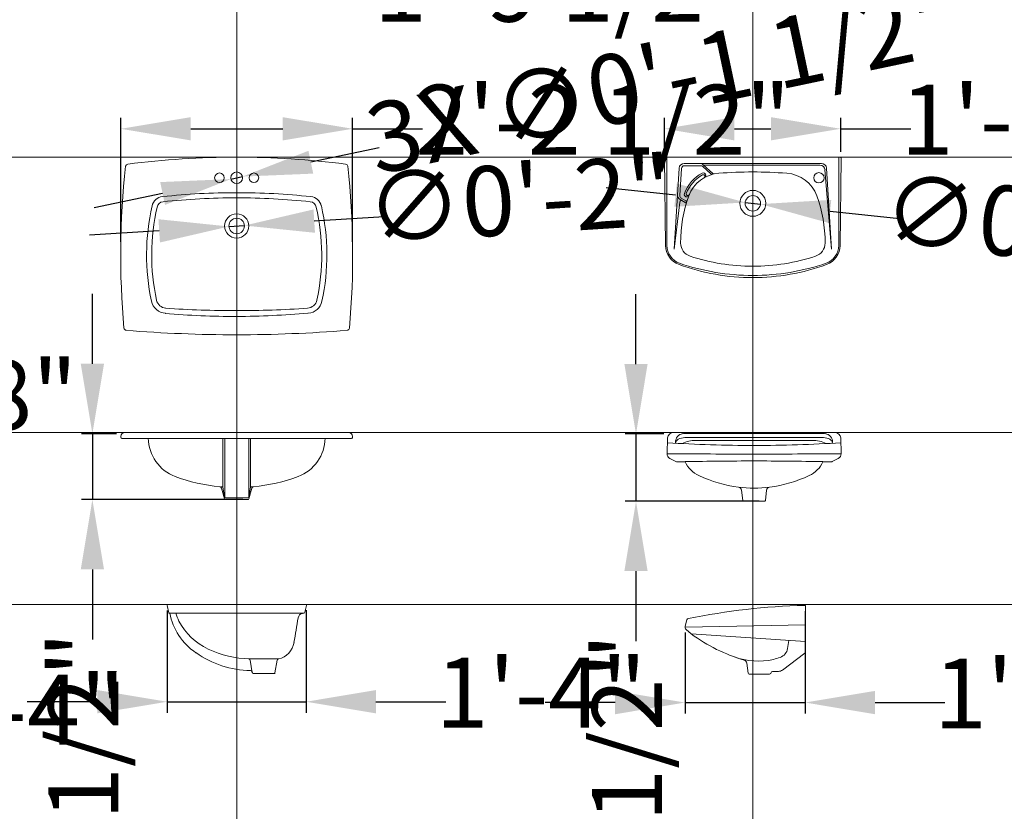
# Model space of a CAD drawing. Units: inches. Extents: x 2138 to 3265, y 2149 to 3392.
# Tile 11 of 13: x 3040 to 3153, y 3164 to 3255. Entities that reach past the tile are written whole.
import ezdxf

# ---------------------------------------------------------------- set-up
doc = ezdxf.new("R2010")
doc.units = ezdxf.units.IN
for name, color, linetype, lineweight in [('A-ANNO-DIMS', 2, 'Continuous', 18), ('A-DETL-GRID', 1, 'Continuous', 13), ('Washbasin-detail', 251, 'Continuous', 13), ('Washbasin-outline', 250, 'Continuous', 20)]:
    doc.layers.add(name, color=color, linetype=linetype, lineweight=lineweight)
doc.styles.get("Standard").update_dxf_attribs({"font": 'arial.ttf'})
doc.dimstyles.new('ISO-25', dxfattribs={"dimtxt": 8, "dimasz": 8, "dimexe": 1.25, "dimexo": 0.625, "dimtad": 0, "dimdec": 1, "dimlunit": 4, "dimtxsty": 'Standard', "dimcen": 2.5, "dimadec": 0, "dimazin": 0, "dimtfac": 1, "dimtdec": 1, "dimtmove": 0, "dimatfit": 3, "dimfxl": 1, "dimarcsym": 0})

# ---------------------------------------------------------------- blocks, each defined once
blk = doc.blocks.new('*D72')
at = {"layer": 'A-ANNO-DIMS', "color": 0, "lineweight": -2, "transparency": 16777216}
for p, q in [((3073.65, 3297.38), (3073.65, 3256.24)), ((3052.31, 3294.65), (3052.31, 3256.24)), ((3060.31, 3257.49), (3065.65, 3257.49)), ((3073.65, 3257.49), (3081.65, 3257.49))]:
    blk.add_line(p, q, dxfattribs=at)
at = {"layer": 'A-ANNO-DIMS', "color": 0, "transparency": 16777216}
for points in [[(3060.31, 3258.82), (3060.31, 3256.15), (3052.31, 3257.49)], [(3065.65, 3258.82), (3065.65, 3256.15), (3073.65, 3257.49)]]:
    blk.add_solid(points, dxfattribs=at)
at = {"layer": 'Defpoints', "color": 0, "transparency": 16777216}
for p in [(3073.65, 3298.01), (3052.31, 3295.28), (3073.65, 3257.49)]:
    blk.add_point(p, dxfattribs=at)
at = {"layer": 'A-ANNO-DIMS', "color": 0, "transparency": 16777216, "insert": (3101.86, 3257.49), "char_height": 8, "attachment_point": 5}
blk.add_mtext('1\'-9 1/2"', dxfattribs=at)
blk = doc.blocks.new('*D85')
at = {"layer": 'A-ANNO-DIMS', "color": 0, "lineweight": -2, "transparency": 16777216}
for p, q in [((2995.75, 3208.1), (2995.75, 3212.02)), ((3015.52, 3208.08), (3015.52, 3212.02)), ((3003.75, 3210.77), (3007.52, 3210.77)), ((3015.52, 3210.77), (3023.52, 3210.77))]:
    blk.add_line(p, q, dxfattribs=at)
at = {"layer": 'A-ANNO-DIMS', "color": 0, "transparency": 16777216}
for points in [[(3003.75, 3212.11), (3003.75, 3209.44), (2995.75, 3210.77)], [(3007.52, 3212.11), (3007.52, 3209.44), (3015.52, 3210.77)]]:
    blk.add_solid(points, dxfattribs=at)
at = {"layer": 'Defpoints', "color": 0, "transparency": 16777216}
for p in [(3015.52, 3210.77), (2995.75, 3207.48), (3015.52, 3207.45)]:
    blk.add_point(p, dxfattribs=at)
at = {"layer": 'A-ANNO-DIMS', "color": 0, "transparency": 16777216, "insert": (3034.4, 3210.77), "char_height": 8, "attachment_point": 5}
blk.add_mtext('1\'-8"', dxfattribs=at)
blk = doc.blocks.new('*D87')
at = {"layer": 'A-ANNO-DIMS', "color": 0, "lineweight": -2, "transparency": 16777216}
for p, q in [((3012.99, 3186.82), (3012.99, 3173.53)), ((2997.1, 3184.61), (2997.1, 3173.53)), ((2989.1, 3174.78), (2981.1, 3174.78)), ((2997.1, 3174.78), (3012.99, 3174.78)), ((3020.99, 3174.78), (3028.99, 3174.78))]:
    blk.add_line(p, q, dxfattribs=at)
at = {"layer": 'A-ANNO-DIMS', "color": 0, "transparency": 16777216}
for points in [[(2989.1, 3176.11), (2989.1, 3173.44), (2997.1, 3174.78)], [(3020.99, 3176.11), (3020.99, 3173.44), (3012.99, 3174.78)]]:
    blk.add_solid(points, dxfattribs=at)
at = {"layer": 'Defpoints', "color": 0, "transparency": 16777216}
for p in [(3012.99, 3187.44), (2997.1, 3185.23), (3012.99, 3174.78)]:
    blk.add_point(p, dxfattribs=at)
at = {"layer": 'A-ANNO-DIMS', "color": 0, "transparency": 16777216, "insert": (3039.87, 3174.78), "char_height": 8, "attachment_point": 5}
blk.add_mtext('1\'-4"', dxfattribs=at)
blk = doc.blocks.new('*D88')
at = {"layer": 'A-ANNO-DIMS', "color": 0, "lineweight": -2, "transparency": 16777216}
for p, q in [((3051.42, 3229.35), (3051.42, 3243.52)), ((3077.95, 3229.35), (3077.95, 3243.52)), ((3059.42, 3242.27), (3069.95, 3242.27)), ((3077.95, 3242.27), (3085.95, 3242.27))]:
    blk.add_line(p, q, dxfattribs=at)
at = {"layer": 'A-ANNO-DIMS', "color": 0, "transparency": 16777216}
for points in [[(3059.42, 3243.6), (3059.42, 3240.94), (3051.42, 3242.27)], [(3069.95, 3243.6), (3069.95, 3240.94), (3077.95, 3242.27)]]:
    blk.add_solid(points, dxfattribs=at)
at = {"layer": 'Defpoints', "color": 0, "transparency": 16777216}
for p in [(3077.95, 3242.27), (3051.42, 3228.73), (3077.95, 3228.73)]:
    blk.add_point(p, dxfattribs=at)
at = {"layer": 'A-ANNO-DIMS', "color": 0, "transparency": 16777216, "insert": (3106.59, 3242.27), "char_height": 8, "attachment_point": 5}
blk.add_mtext('2\'-2 1/2"', dxfattribs=at)
blk = doc.blocks.new('*D89')
at = {"layer": 'A-ANNO-DIMS', "color": 0, "lineweight": -2, "transparency": 16777216}
for p, q in [((3048.17, 3215.38), (3048.17, 3223.38)), ((3050.93, 3207.38), (3046.92, 3207.38)), ((3048.17, 3207.38), (3048.17, 3199.85)), ((3065.38, 3199.85), (3046.92, 3199.85)), ((3048.17, 3191.85), (3048.17, 3183.85))]:
    blk.add_line(p, q, dxfattribs=at)
at = {"layer": 'A-ANNO-DIMS', "color": 0, "transparency": 16777216}
for points in [[(3046.84, 3215.38), (3049.5, 3215.38), (3048.17, 3207.38)], [(3046.84, 3191.85), (3049.5, 3191.85), (3048.17, 3199.85)]]:
    blk.add_solid(points, dxfattribs=at)
at = {"layer": 'Defpoints', "color": 0, "transparency": 16777216}
for p in [(3051.56, 3207.38), (3048.17, 3199.85), (3066, 3199.85)]:
    blk.add_point(p, dxfattribs=at)
at = {"layer": 'A-ANNO-DIMS', "color": 0, "transparency": 16777216, "insert": (3048.17, 3163.27), "char_height": 8, "attachment_point": 5, "rotation": 90}
blk.add_mtext('0\'-7 1/2"', dxfattribs=at)
blk = doc.blocks.new('*D90')
at = {"layer": 'A-ANNO-DIMS', "color": 0, "lineweight": -2, "transparency": 16777216}
for p, q in [((3056.72, 3187.14), (3056.72, 3175.46)), ((3072.62, 3187.18), (3072.62, 3175.46)), ((3048.72, 3176.71), (3040.72, 3176.71)), ((3056.72, 3176.71), (3072.62, 3176.71)), ((3080.62, 3176.71), (3088.62, 3176.71))]:
    blk.add_line(p, q, dxfattribs=at)
at = {"layer": 'A-ANNO-DIMS', "color": 0, "transparency": 16777216}
for points in [[(3048.72, 3178.05), (3048.72, 3175.38), (3056.72, 3176.71)], [(3080.62, 3178.05), (3080.62, 3175.38), (3072.62, 3176.71)]]:
    blk.add_solid(points, dxfattribs=at)
at = {"layer": 'Defpoints', "color": 0, "transparency": 16777216}
for p in [(3056.72, 3187.77), (3072.62, 3187.8), (3072.62, 3176.71)]:
    blk.add_point(p, dxfattribs=at)
at = {"layer": 'A-ANNO-DIMS', "color": 0, "transparency": 16777216, "insert": (3099.5, 3176.71), "char_height": 8, "attachment_point": 5}
blk.add_mtext('1\'-4"', dxfattribs=at)
blk = doc.blocks.new('*D91')
at = {"layer": 'A-ANNO-DIMS', "color": 0, "lineweight": -2, "transparency": 16777216}
for p, q in [((3113.64, 3239.59), (3113.64, 3243.52)), ((3133.8, 3239.62), (3133.8, 3243.52)), ((3121.64, 3242.27), (3125.8, 3242.27)), ((3133.8, 3242.27), (3141.8, 3242.27))]:
    blk.add_line(p, q, dxfattribs=at)
at = {"layer": 'A-ANNO-DIMS', "color": 0, "transparency": 16777216}
for points in [[(3121.64, 3243.6), (3121.64, 3240.94), (3113.64, 3242.27)], [(3125.8, 3243.6), (3125.8, 3240.94), (3133.8, 3242.27)]]:
    blk.add_solid(points, dxfattribs=at)
at = {"layer": 'Defpoints', "color": 0, "transparency": 16777216}
for p in [(3133.8, 3242.27), (3113.64, 3238.97), (3133.8, 3239)]:
    blk.add_point(p, dxfattribs=at)
at = {"layer": 'A-ANNO-DIMS', "color": 0, "transparency": 16777216, "insert": (3152.69, 3242.27), "char_height": 8, "attachment_point": 5}
blk.add_mtext('1\'-8"', dxfattribs=at)
blk = doc.blocks.new('*D92')
at = {"layer": 'A-ANNO-DIMS', "color": 0, "lineweight": -2, "transparency": 16777216}
for p, q in [((3110.37, 3215.35), (3110.37, 3223.35)), ((3113.57, 3207.35), (3109.12, 3207.35)), ((3110.37, 3207.35), (3110.37, 3199.66)), ((3124.47, 3199.66), (3109.12, 3199.66)), ((3110.37, 3191.66), (3110.37, 3183.66))]:
    blk.add_line(p, q, dxfattribs=at)
at = {"layer": 'A-ANNO-DIMS', "color": 0, "transparency": 16777216}
for points in [[(3109.04, 3215.35), (3111.7, 3215.35), (3110.37, 3207.35)], [(3109.04, 3191.66), (3111.7, 3191.66), (3110.37, 3199.66)]]:
    blk.add_solid(points, dxfattribs=at)
at = {"layer": 'Defpoints', "color": 0, "transparency": 16777216}
for p in [(3114.19, 3207.35), (3110.37, 3199.66), (3125.1, 3199.66)]:
    blk.add_point(p, dxfattribs=at)
at = {"layer": 'A-ANNO-DIMS', "color": 0, "transparency": 16777216, "insert": (3110.37, 3163.08), "char_height": 8, "attachment_point": 5, "rotation": 90}
blk.add_mtext('0\'-7 1/2"', dxfattribs=at)
blk = doc.blocks.new('*D93')
at = {"layer": 'A-ANNO-DIMS', "color": 0, "lineweight": -2, "transparency": 16777216}
for p, q in [((3129.72, 3187.08), (3129.72, 3175.37)), ((3115.98, 3184.63), (3115.98, 3175.37)), ((3107.98, 3176.62), (3099.98, 3176.62)), ((3115.98, 3176.62), (3129.72, 3176.62)), ((3137.72, 3176.62), (3145.72, 3176.62))]:
    blk.add_line(p, q, dxfattribs=at)
at = {"layer": 'A-ANNO-DIMS', "color": 0, "transparency": 16777216}
for points in [[(3107.98, 3177.95), (3107.98, 3175.28), (3115.98, 3176.62)], [(3137.72, 3177.95), (3137.72, 3175.28), (3129.72, 3176.62)]]:
    blk.add_solid(points, dxfattribs=at)
at = {"layer": 'Defpoints', "color": 0, "transparency": 16777216}
for p in [(3129.72, 3187.71), (3115.98, 3185.26), (3129.72, 3176.62)]:
    blk.add_point(p, dxfattribs=at)
at = {"layer": 'A-ANNO-DIMS', "color": 0, "transparency": 16777216, "insert": (3165.92, 3176.62), "char_height": 8, "attachment_point": 5}
blk.add_mtext('1\'-1 1/2"', dxfattribs=at)
blk = doc.blocks.new('*D125')
at = {"layer": 'A-ANNO-DIMS', "color": 0, "lineweight": -2, "transparency": 16777216}
for p, q in [((3080.99, 3240.1), (3073.17, 3238.45)), ((3064.03, 3236.52), (3065.34, 3236.8)), ((3056.2, 3234.87), (3048.37, 3233.21))]:
    blk.add_line(p, q, dxfattribs=at)
at = {"layer": 'A-ANNO-DIMS', "color": 0, "transparency": 16777216}
for points in [[(3072.89, 3239.75), (3073.44, 3237.14), (3065.34, 3236.8)], [(3055.93, 3236.17), (3056.48, 3233.56), (3064.03, 3236.52)]]:
    blk.add_solid(points, dxfattribs=at)
at = {"layer": 'Defpoints', "color": 0, "transparency": 16777216}
for p in [(3065.34, 3236.8), (3064.03, 3236.52)]:
    blk.add_point(p, dxfattribs=at)
at = {"layer": 'A-ANNO-DIMS', "color": 0, "transparency": 16777216, "insert": (3113.58, 3246.98), "char_height": 8, "attachment_point": 5, "rotation": 11.9181}
blk.add_mtext('3X ∅0\'-1 1/2"', dxfattribs=at)
blk = doc.blocks.new('*D126')
at = {"layer": 'A-ANNO-DIMS', "color": 0, "lineweight": -2, "transparency": 16777216}
for p, q in [((3081.54, 3232.21), (3073.55, 3231.7)), ((3063.8, 3231.09), (3065.57, 3231.2)), ((3055.81, 3230.59), (3047.83, 3230.08))]:
    blk.add_line(p, q, dxfattribs=at)
at = {"layer": 'A-ANNO-DIMS', "color": 0, "transparency": 16777216}
for points in [[(3073.47, 3233.04), (3073.64, 3230.37), (3065.57, 3231.2)], [(3055.73, 3231.92), (3055.9, 3229.26), (3063.8, 3231.09)]]:
    blk.add_solid(points, dxfattribs=at)
at = {"layer": 'Defpoints', "color": 0, "transparency": 16777216}
for p in [(3063.8, 3231.09), (3065.57, 3231.2)]:
    blk.add_point(p, dxfattribs=at)
at = {"layer": 'A-ANNO-DIMS', "color": 0, "transparency": 16777216, "insert": (3097.11, 3233.19), "char_height": 8, "attachment_point": 5, "rotation": 3.6089}
blk.add_mtext('∅0\'-2"', dxfattribs=at)
blk = doc.blocks.new('*D127')
at = {"layer": 'A-ANNO-DIMS', "color": 0, "lineweight": -2, "transparency": 16777216}
for p, q in [((3114.9, 3234.67), (3106.94, 3235.51)), ((3122.86, 3233.84), (3124.62, 3233.65)), ((3140.53, 3231.98), (3132.58, 3232.81))]:
    blk.add_line(p, q, dxfattribs=at)
at = {"layer": 'A-ANNO-DIMS', "color": 0, "transparency": 16777216}
for points in [[(3115.04, 3236), (3114.76, 3233.35), (3122.86, 3233.84)], [(3132.71, 3234.14), (3132.44, 3231.49), (3124.62, 3233.65)]]:
    blk.add_solid(points, dxfattribs=at)
at = {"layer": 'Defpoints', "color": 0, "transparency": 16777216}
for p in [(3122.86, 3233.84), (3124.62, 3233.65)]:
    blk.add_point(p, dxfattribs=at)
at = {"layer": 'A-ANNO-DIMS', "color": 0, "transparency": 16777216, "insert": (3156.06, 3230.35), "char_height": 8, "attachment_point": 5, "rotation": 353.9986}
blk.add_mtext('∅0\'-2"', dxfattribs=at)

msp = doc.modelspace()

# ---------------------------------------------------------------- linework, layer by layer
at = {"layer": 'A-DETL-GRID'}
for p, q in [((3064.68, 3239.02), (3064.68, 3370.91)), ((3123.74, 3239.02), (3123.74, 3370.91)), ((2828.46, 3239.02), (3241.85, 3239.02)), ((2828.46, 3239.02), (3241.85, 3239.02)), ((3064.68, 3148.47), (3064.68, 3239.02)), ((3123.74, 3148.47), (3123.74, 3239.02)), ((2828.46, 3207.52), (3241.85, 3207.52)), ((2828.46, 3187.84), (3241.85, 3187.84))]:
    msp.add_line(p, q, dxfattribs=at)
at = {"layer": 'Washbasin-detail'}
for p, q in [((3113.9, 3239.02), (3113.9, 3228.9)), ((3133.58, 3239.02), (3133.58, 3228.9)), ((3123.74, 3238.31), (3115.9, 3238.31)), ((3117.79, 3238.04), (3115.9, 3238.04)), ((3118, 3237.95), (3118.93, 3237.1)), ((3118.07, 3238.16), (3119.16, 3237.16)), ((3131.41, 3238.11), (3118.11, 3238.11)), ((3123.74, 3238.31), (3131.58, 3238.31)), ((3114.75, 3228.51), (3115.31, 3237.76)), ((3115.39, 3234.63), (3115.58, 3237.74)), ((3132.73, 3228.51), (3131.99, 3237.57)), ((3132.73, 3228.51), (3132.17, 3237.76)), ((3115.38, 3233.89), (3114.75, 3228.51)), ((3115.42, 3234.19), (3116.01, 3233.85)), ((3115.55, 3234.34), (3116.07, 3234.04)), ((3123.88, 3207.41), (3115.91, 3207.41)), ((3123.88, 3207.41), (3131.85, 3207.41)), ((3063.11, 3206.85), (3063.11, 3201.3)), ((3063.31, 3206.85), (3063.31, 3200.1)), ((3066.06, 3206.85), (3066.06, 3200.1)), ((3066.25, 3206.85), (3066.25, 3201.3)), ((3114.89, 3206.42), (3114.89, 3206.29)), ((3123.88, 3206.93), (3115.95, 3206.93)), ((3117.21, 3206.62), (3130.55, 3206.62)), ((3123.88, 3206.93), (3131.81, 3206.93)), ((3062.82, 3201.29), (3063.11, 3201.29)), ((3063.29, 3199.93), (3062.96, 3201.13)), ((3063.11, 3201.28), (3063.29, 3200.14)), ((3066.25, 3201.28), (3066.07, 3200.14)), ((3066.08, 3199.93), (3066.41, 3201.13)), ((3066.55, 3201.29), (3066.25, 3201.29)), ((3063.4, 3199.85), (3064.68, 3199.85)), ((3063.41, 3200.04), (3064.69, 3200.04)), ((3063.41, 3200.04), (3064.69, 3200.04)), ((3065.95, 3200.04), (3064.68, 3200.04)), ((3065.95, 3200.04), (3064.68, 3200.04)), ((3065.97, 3199.85), (3064.68, 3199.85)), ((3129.76, 3185.5), (3115.98, 3185.26)), ((3116.69, 3184.47), (3129.76, 3183.61)), ((3127.87, 3183.73), (3127.72, 3182.8))]:
    msp.add_line(p, q, dxfattribs=at)
for centre, radius in [((3062.71, 3236.66), 0.551), ((3064.68, 3236.66), 0.669), ((3066.65, 3236.66), 0.551), ((3131.3, 3236.66), 0.591)]:
    msp.add_circle(centre, radius, dxfattribs=at)
for centre, radius, start, end in [((3115.9, 3237.72), 0.591, 90, 176.5501), ((3115.9, 3237.72), 0.315, 90, 176.5501), ((3117.67, 3237.72), 0.591, 47.5081, 90), ((3117.79, 3237.72), 0.315, 47.5081, 90), ((3131.41, 3237.52), 0.591, 4.6212, 90), ((3131.58, 3237.72), 0.591, 3.4499, 90), ((3120.14, 3233.25), 4.53, 119.1249, 158.9278), ((3120.14, 3233.25), 4.33, 119.974, 157.8804), ((3118.08, 3236.95), 0.289, 298.884, 120.9504), ((3118.07, 3236.83), 0.19, 299.8578, 119.974), ((3119.06, 3237.25), 0.197, 227.5081, 284.9221), ((3119.29, 3237.3), 0.197, 227.5081, 281.6214), ((3115.71, 3234.7), 0.591, 176.5501, 239.9947), ((3115.71, 3234.61), 0.315, 176.5501, 239.9947), ((3116.18, 3234.76), 0.287, 157.239, 339.7253), ((3116.3, 3234.81), 0.189, 157.8804, 337.9006), ((3123.74, 3233.74), 1.48, 90, 270), ((3123.74, 3233.74), 0.886, 90, 270), ((3123.74, 3233.74), 1.48, 270, 90), ((3123.74, 3233.74), 0.886, 270, 90), ((3079.63, 3227.83), 24.67, 167.1604, 192.0964), ((3056.34, 3233.14), 0.787, 96.1416, 167.1604), ((3064.68, 3155.63), 78.74, 90, 96.1416), ((3064.68, 3155.63), 78.74, 83.8584, 90), ((3073.02, 3233.14), 0.787, 12.8396, 83.8584), ((3049.74, 3227.83), 24.67, 347.9251, 12.8396), ((3115.58, 3233.87), 0.197, 59.9947, 173.2749), ((3115.91, 3233.68), 0.197, 343.7163, 59.9947), ((3115.97, 3233.87), 0.197, 342.9893, 59.9947), ((3064.68, 3231.15), 1.38, 90, 270), ((3064.68, 3231.15), 1.38, 270, 90), ((3064.68, 3231.15), 0.886, 90, 270), ((3064.68, 3231.15), 0.886, 270, 90), ((3116.12, 3228.96), 2.22, 180.7821, 249.7803), ((3131.36, 3228.96), 2.22, 290.2197, 359.2179), ((3123.74, 3251.47), 25.98, 251.1623, 270), ((3123.74, 3251.47), 25.98, 270, 288.8377), ((3056.66, 3222.92), 1.18, 192.0749, 266.0653), ((3072.71, 3222.92), 1.18, 273.9347, 347.9251), ((3064.68, 3339.57), 118.11, 266.049, 270), ((3064.68, 3339.57), 118.11, 270, 273.9347), ((3115.91, 3206.22), 1.18, 90, 99.548), ((3131.85, 3206.22), 1.18, 80.452, 90), ((3059.29, 3206.91), 4.72, 180.6352, 249.5876), ((3070.07, 3206.91), 4.72, 290.4124, 359.3648), ((3115.87, 3206.42), 0.984, 99.548, 180), ((3115.48, 3206.22), 0.591, 118.4442, 173.4004), ((3115.95, 3205.36), 1.57, 90, 118.4442), ((3117.21, 3203.16), 3.46, 90, 116.7072), ((3130.55, 3203.16), 3.46, 63.2928, 90), ((3131.81, 3205.36), 1.57, 61.5558, 90), ((3131.88, 3206.42), 0.984, 0, 80.452), ((3132.28, 3206.22), 0.591, 6.5996, 61.5558), ((3123.88, 4523.81), 1318.76, 269.56724, 270), ((3123.88, 4523.81), 1318.76, 270, 270.43276), ((3064.65, 3221.3), 20.08, 249.5876, 264.5822), ((3064.72, 3221.3), 20.08, 275.4178, 290.4124), ((3062.73, 3201.07), 0.236, 15.2242, 84.5822), ((3063.23, 3201.3), 0.118, 180, 188.9509), ((3066.13, 3201.3), 0.118, 351.0491, 0), ((3066.63, 3201.07), 0.236, 95.4178, 164.7758), ((3063.41, 3200.16), 0.118, 188.9509, 270), ((3063.4, 3199.96), 0.118, 195.2242, 270), ((3065.95, 3200.16), 0.118, 270, 351.0491), ((3065.97, 3199.96), 0.118, 270, 344.7758), ((3063.98, 3188.2), 7.09, 190.9924, 235.973), ((3126.43, 3183.01), 1.3, 290.1504, 350.6185), ((3066.42, 3191.3), 11.02, 234.5166, 269.1523), ((3124.38, 3189.5), 8.14, 250.1072, 282.2031), ((3124.06, 3189.48), 8.19, 284.427, 290.1504)]:
    msp.add_arc(centre, radius, start, end, dxfattribs=at)
at = {"layer": 'Washbasin-outline'}
for p, q in [((3051.89, 3207.52), (3064.68, 3207.52)), ((3077.47, 3207.52), (3064.68, 3207.52)), ((3051.42, 3207.05), (3051.42, 3206.97)), ((3051.54, 3206.85), (3064.69, 3206.85)), ((3077.83, 3206.85), (3064.68, 3206.85)), ((3077.95, 3207.05), (3077.95, 3206.97)), ((3056.9, 3186.88), (3056.71, 3187.72)), ((3056.83, 3187.84), (3072.54, 3187.84)), ((3072.66, 3187.72), (3072.48, 3186.96)), ((3056.93, 3186.85), (3057.03, 3186.85)), ((3057.03, 3186.85), (3072.4, 3186.85)), ((3072.2, 3186.81), (3072.36, 3186.84)), ((3066.17, 3181.62), (3069.52, 3181.62)), ((3066.22, 3181.45), (3066.47, 3180.03)), ((3069.32, 3181.45), (3069.06, 3180.03)), ((3066.48, 3180.02), (3066.44, 3180.14)), ((3066.55, 3179.96), (3068.99, 3179.96))]:
    msp.add_line(p, q, dxfattribs=at)
for points in [[(3115.3, 3226.74, -0.310499), (3113.76, 3228.93), (3113.62, 3238.9, -0.418217), (3113.74, 3239.02), (3123.74, 3239.02), (3133.74, 3239.02, -0.418217), (3133.86, 3238.9), (3133.72, 3228.93, -0.310499), (3132.17, 3226.74, -0.088455), (3123.74, 3225.24, -0.088455)], [(3123.88, 3207.52), (3114.66, 3207.52, 0.377881), (3113.96, 3206.9), (3113.92, 3205.09, 0.28521), (3114.23, 3204.56), (3114.93, 3204.19, 0.126322), (3115.06, 3204.16, -0.000566), (3116, 3204.18, 0.184451), (3117.57, 3202.58, 0.073376), (3122.1, 3201.26, -0.338761), (3122.44, 3200.92), (3122.59, 3199.75, 0.377345), (3122.7, 3199.65), (3123.88, 3199.65), (3125.05, 3199.65, 0.377345), (3125.17, 3199.75), (3125.32, 3200.92, -0.338761), (3125.66, 3201.26, 0.073376), (3130.18, 3202.58, 0.184451), (3131.76, 3204.18, -0.000566), (3132.7, 3204.16, 0.126322), (3132.82, 3204.19), (3133.52, 3204.56, 0.28521), (3133.84, 3205.09), (3133.8, 3206.9, 0.377881), (3133.1, 3207.52)]]:
    msp.add_lwpolyline(points, format="xyb", close=True, dxfattribs=at)
msp.add_lwpolyline([(3126.08, 3180.18), (3126.66, 3180.18), (3126.08, 3180.18, 0.335437), (3125.78, 3179.95, -0.335437), (3125.66, 3179.87), (3123.31, 3179.87, -0.377345), (3123.19, 3179.97), (3123.04, 3181.14, 0.297687), (3122.76, 3181.47, -0.086663), (3116.69, 3184.47), (3116.12, 3184.96, -0.289634), (3115.99, 3185.36), (3116.18, 3186.07, -0.28455), (3116.36, 3186.24, -0.042482), (3129.64, 3187.74, -0.422344), (3129.76, 3187.62), (3129.76, 3182.41, -0.236068), (3129.68, 3182.25), (3127.13, 3180.34, -0.162278), (3126.66, 3180.18)], format="xyb", dxfattribs=at)
for centre, radius, start, end in [((3064.68, 3140.59), 98.43, 90, 97.2742), ((3064.68, 3140.59), 98.43, 82.7258, 90), ((3143.98, 3227.76), 92.57, 173.6587, 185.1425), ((3052.26, 3237.95), 0.276, 97.2742, 173.6587), ((3077.11, 3237.95), 0.276, 6.3413, 82.7258), ((2985.38, 3227.76), 92.57, 354.8575, 6.3413), ((3120.12, 3233.25), 3.94, 94.015, 159.961), ((3123.98, 3178.27), 59.06, 90.2363, 94.015), ((3123.49, 3178.27), 59.06, 85.985, 89.7637), ((3127.35, 3233.25), 3.94, 20.039, 85.985), ((3056.34, 3233.14), 1.38, 96.1416, 167.1604), ((3064.68, 3155.63), 79.33, 90, 96.1416), ((3064.68, 3155.63), 79.33, 83.8584, 90), ((3073.02, 3233.14), 1.38, 12.8396, 83.8584), ((3131.22, 3229.21), 15.75, 159.961, 180.0563), ((3116.26, 3229.21), 15.75, 359.9437, 20.039), ((3079.63, 3227.83), 25.26, 167.1604, 192.0749), ((3049.74, 3227.83), 25.26, 347.9251, 12.8396), ((3117.05, 3229.19), 1.57, 180, 251.6504), ((3130.43, 3229.19), 1.57, 288.3496, 0), ((3123.74, 3249.37), 22.83, 251.6504, 270), ((3123.74, 3249.37), 22.83, 270, 288.3496), ((3056.66, 3222.92), 1.77, 192.0749, 266.0653), ((3072.71, 3222.92), 1.77, 275.0575, 347.9251), ((3064.68, 3313.58), 92.79, 264.9425, 270), ((3063.54, 3339.49), 118.7, 270.5523, 274.5052), ((3072.71, 3222.92), 1.77, 273.9347, 275.0575), ((3052.06, 3219.49), 0.276, 185.1425, 265.3953), ((3064.68, 3376.18), 157.48, 265.3953, 270), ((3064.68, 3376.18), 157.48, 270, 274.6047), ((3077.3, 3219.49), 0.276, 274.6047, 354.8575), ((3051.89, 3207.05), 0.472, 90, 180), ((3077.47, 3207.05), 0.472, 0, 90), ((3051.54, 3206.97), 0.118, 180, 270), ((3077.83, 3206.97), 0.118, 270, 0), ((3123.88, 3358.99), 152.96, 266.2773, 270.0006), ((3123.88, 3358.99), 152.96, 269.9994, 273.7227), ((3123.88, 2789.3), 414.96, 90, 91.0879), ((3123.88, 2789.3), 414.96, 88.9121, 90), ((3123.88, 3215.22), 14.07, 262.7274, 277.2726), ((3056.83, 3187.72), 0.118, 90, 180), ((3072.54, 3187.72), 0.118, 0, 90), ((3056.94, 3186.89), 0.0394, 192.8043, 256.7595), ((3062.53, 3188.3), 5.04, 196.7804, 207.8951), ((2876.94, 3217.46), 197.24, 350.0842, 350.9161), ((3072.3, 3186.23), 0.591, 100.008, 170.9161), ((3072.33, 3186.99), 0.157, 280.008, 347.1957), ((3064.62, 3189.41), 7.4, 207.8951, 244.3062), ((3066.33, 3192.96), 11.34, 244.3062, 269.213), ((3068.92, 3183.9), 2.36, 283.4865, 350.0842), ((3066.03, 3181.41), 0.197, 10.1247, 76.5135), ((3069.51, 3181.41), 0.197, 103.4865, 169.8753), ((3066.25, 3180.08), 0.197, 17.354, 89.1523), ((3066.55, 3180.04), 0.0787, 197.354, 270), ((3068.99, 3180.04), 0.0787, 270, 349.8753)]:
    msp.add_arc(centre, radius, start, end, dxfattribs=at)

# ---------------------------------------------------------------- dimensions: what is measured, and where the dimension line sits
at = {"layer": 'A-ANNO-DIMS'}
for base, p1, p2, picture, middle in [((3073.65, 3257.49), (3052.31, 3295.28), (3073.65, 3298.01), '*D72', (3101.86, 3257.49)), ((3077.95, 3242.27), (3051.42, 3228.73), (3077.95, 3228.73), '*D88', (3106.59, 3242.27)), ((3133.8, 3242.27), (3113.64, 3238.97), (3133.8, 3239), '*D91', (3152.69, 3242.27)), ((3015.52, 3210.77), (2995.75, 3207.48), (3015.52, 3207.45), '*D85', (3034.4, 3210.77)), ((3129.72, 3176.62), (3115.98, 3185.26), (3129.72, 3187.71), '*D93', (3165.92, 3176.62)), ((3012.99, 3174.78), (2997.1, 3185.23), (3012.99, 3187.44), '*D87', (3039.87, 3174.78)), ((3072.62, 3176.71), (3056.72, 3187.77), (3072.62, 3187.8), '*D90', (3099.5, 3176.71))]:
    dim = msp.add_linear_dim(base=base, p1=p1, p2=p2, dimstyle='ISO-25', override={"dimdec": 1, "dimlfac": 1, "dimrnd": 0, "dimzin": 1, "dimdsep": 46, "dimlunit": 4, "dimfrac": 2}, dxfattribs=at)
    dim.commit()
    dim.dimension.update_dxf_attribs({"geometry": picture, "text_midpoint": middle})
dim = msp.add_diameter_dim_2p(p1=(3064.03, 3236.52), p2=(3065.34, 3236.8), text='3X <>', dimstyle='ISO-25', override={"dimdec": 1, "dimlfac": 1, "dimrnd": 0, "dimzin": 1, "dimdsep": 46, "dimlunit": 4, "dimfrac": 2}, dxfattribs=at)
dim.commit()
dim.dimension.update_dxf_attribs({"geometry": '*D125', "text_midpoint": (3113.58, 3246.98), "dimtype": 163})
for p1, p2, picture, middle in [((3063.8, 3231.09), (3065.57, 3231.2), '*D126', (3097.11, 3233.19)), ((3122.86, 3233.84), (3124.62, 3233.65), '*D127', (3156.06, 3230.35))]:
    dim = msp.add_diameter_dim_2p(p1=p1, p2=p2, dimstyle='ISO-25', override={"dimdec": 1, "dimlfac": 1, "dimrnd": 0, "dimzin": 1, "dimdsep": 46, "dimlunit": 4, "dimfrac": 2}, dxfattribs=at)
    dim.commit()
    dim.dimension.update_dxf_attribs({"geometry": picture, "text_midpoint": middle})
for base, p1, p2, picture, middle in [((3048.17, 3199.85), (3051.56, 3207.38), (3066, 3199.85), '*D89', (3048.17, 3163.27)), ((3110.37, 3199.66), (3114.19, 3207.35), (3125.1, 3199.66), '*D92', (3110.37, 3163.08))]:
    dim = msp.add_linear_dim(base=base, p1=p1, p2=p2, angle=90, dimstyle='ISO-25', override={"dimdec": 1, "dimlfac": 1, "dimrnd": 0, "dimzin": 1, "dimdsep": 46, "dimlunit": 4, "dimfrac": 2}, dxfattribs=at)
    dim.commit()
    dim.dimension.update_dxf_attribs({"geometry": picture, "text_midpoint": middle})

doc.saveas('drawing.dxf')
